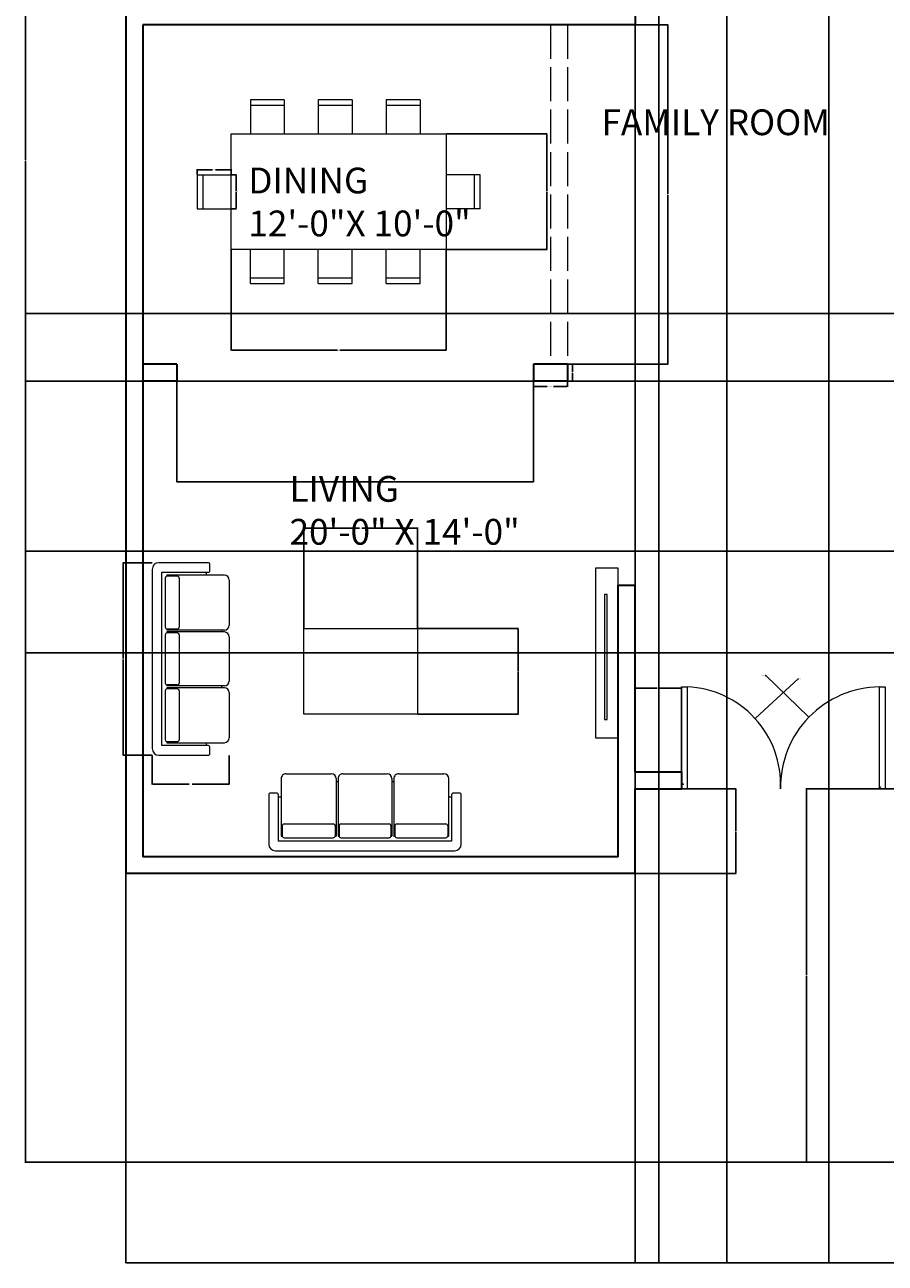
# Model space of a CAD drawing. Units: inches. Extents: x 4468 to 4972, y 2758 to 3538.
# Tile 1 of 4: x 4468 to 4772, y 2758 to 3196. Entities that reach past the tile are written whole.
import ezdxf

# ---------------------------------------------------------------- set-up
doc = ezdxf.new("R2010")
doc.units = ezdxf.units.IN
doc.linetypes.add('ACAD_ISO02W100', pattern=[15, 12, -3])
for name, color, linetype, lineweight in [('A-ANNO-DIMS', 2, 'Continuous', 18), ('A-AREA-IDEN', 7, 'Continuous', 18), ('A-COLS', 7, 'Continuous', 35), ('A-DOOR', 4, 'Continuous', 18), ('A-EQPM', 8, 'Continuous', 18), ('A-FLOR-OVHD', 8, 'ACAD_ISO02W100', 13), ('A-FURN', 8, 'Continuous', 15), ('A-WALL', 7, 'Continuous', 35)]:
    doc.layers.add(name, color=color, linetype=linetype, lineweight=lineweight)
doc.styles.get("Standard").update_dxf_attribs({"font": 'arial.ttf'})
doc.dimstyles.get("Standard").update_dxf_attribs({"dimtxt": 0.18, "dimasz": 0.18, "dimexe": 0.18, "dimexo": 0.0625, "dimgap": 0.09, "dimtad": 0, "dimtih": 1, "dimtoh": 1, "dimdec": 4, "dimzin": 0, "dimdsep": 46, "dimtxsty": 'Standard', "dimcen": 0.09, "dimadec": 0, "dimazin": 0, "dimtfac": 1, "dimtdec": 4, "dimtofl": 0, "dimtmove": 0, "dimatfit": 3, "dimfxl": 1, "dimtolj": 1, "dimtzin": 0, "dimarcsym": 0})

# ---------------------------------------------------------------- blocks, each defined once
blk = doc.blocks.new('A$C06FC73D7')
for p, q in [((1.93, 0.8), (0.07, 0.8)), ((0, 0.73), (0, 0.22)), ((0.1, 0.22), (0.1, 0.7)), ((0.1, 0.7), (1.9, 0.7)), ((0.13, 0.648), (0.13, 0.05)), ((0.14, 0.648), (0.13, 0.648)), ((0.14, 0.54), (0.14, 0.644)), ((0.67, 0.664), (0.16, 0.664)), ((0.7, 0.648), (0.69, 0.648)), ((0.69, 0.54), (0.69, 0.644)), ((0.7, 0.05), (0.7, 0.648)), ((0.72, 0.05), (0.72, 0.648)), ((0.73, 0.648), (0.72, 0.648)), ((0.73, 0.54), (0.73, 0.644)), ((1.25, 0.664), (0.75, 0.664)), ((1.28, 0.648), (1.27, 0.648)), ((1.27, 0.54), (1.27, 0.644)), ((1.28, 0.05), (1.28, 0.648)), ((1.3, 0.05), (1.3, 0.648)), ((1.31, 0.648), (1.3, 0.648)), ((1.31, 0.54), (1.31, 0.644)), ((1.84, 0.664), (1.33, 0.664)), ((1.87, 0.648), (1.86, 0.648)), ((1.86, 0.54), (1.86, 0.644)), ((1.87, 0.05), (1.87, 0.648)), ((1.9, 0.7), (1.9, 0.22)), ((2, 0.22), (2, 0.73)), ((0.67, 0.52), (0.16, 0.52)), ((1.25, 0.52), (0.75, 0.52)), ((1.84, 0.52), (1.33, 0.52)), ((0.02, 0.2), (0.08, 0.2)), ((0.13, 0.24), (0.1, 0.24)), ((1.9, 0.24), (1.87, 0.24)), ((1.92, 0.2), (1.98, 0.2)), ((0.65, 0), (0.18, 0)), ((0.72, 0.08), (0.7, 0.08)), ((1.23, 0), (0.77, 0)), ((1.3, 0.08), (1.28, 0.08)), ((1.82, 0), (1.35, 0))]:
    blk.add_line(p, q)
for centre, radius, start, end in [((0.07, 0.73), 0.07, 90, 180), ((1.93, 0.73), 0.07, 0, 90), ((0.16, 0.644), 0.02, 90, 180), ((0.67, 0.644), 0.02, 0, 90), ((0.75, 0.644), 0.02, 90, 180), ((1.25, 0.644), 0.02, 0, 90), ((1.33, 0.644), 0.02, 90, 180), ((1.84, 0.644), 0.02, 0, 90), ((0.16, 0.54), 0.02, 180, 270), ((0.67, 0.54), 0.02, 270, 0), ((0.75, 0.54), 0.02, 180, 270), ((1.25, 0.54), 0.02, 270, 0), ((1.33, 0.54), 0.02, 180, 270), ((1.84, 0.54), 0.02, 270, 0), ((0.02, 0.22), 0.02, 180, 270), ((0.08, 0.22), 0.02, 270, 0), ((1.92, 0.22), 0.02, 180, 270), ((1.98, 0.22), 0.02, 270, 0), ((0.18, 0.05), 0.05, 180, 270), ((0.65, 0.05), 0.05, 270, 0), ((0.77, 0.05), 0.05, 180, 270), ((1.23, 0.05), 0.05, 270, 0), ((1.35, 0.05), 0.05, 180, 270), ((1.82, 0.05), 0.05, 270, 0)]:
    blk.add_arc(centre, radius, start, end)
blk = doc.blocks.new('CHAIR-DINING')
for p, q in [((0, 0), (0, 12)), ((12, 0), (12, 12)), ((0, 2), (12, 2)), ((0, 0), (12, 0))]:
    blk.add_line(p, q)
blk = doc.blocks.new('COL-12X6')
for p, q in [((12, 6), (0, 6)), ((0, 6), (0, 0)), ((12, 6), (12, 0)), ((12, 0), (0, 0))]:
    blk.add_line(p, q)
blk = doc.blocks.new('DOOR-LEAF-36IN')
for p, q in [((0, 0), (0, 36)), ((0, 36), (2, 36)), ((2, 36), (2, 0)), ((2, 0), (0, 0))]:
    blk.add_line(p, q)
blk = doc.blocks.new('*D15')
at = {"layer": 'A-ANNO-DIMS', "color": 0, "lineweight": -2, "transparency": 16777216}
for p, q in [((4541.41, 3143.14), (4543.32, 3143.14)), ((4543.14, 3142.96), (4543.14, 3137.32)), ((4543.14, 3131.32), (4543.14, 3136.96)), ((4541.41, 3131.14), (4543.32, 3131.14))]:
    blk.add_line(p, q, dxfattribs=at)
at = {"layer": 'A-ANNO-DIMS', "color": 0, "transparency": 16777216}
for points in [[(4543.11, 3142.96), (4543.17, 3142.96), (4543.14, 3143.14)], [(4543.11, 3131.32), (4543.17, 3131.32), (4543.14, 3131.14)]]:
    blk.add_solid(points, dxfattribs=at)
at = {"layer": 'Defpoints', "color": 0, "transparency": 16777216}
for p in [(4541.34, 3143.14), (4541.34, 3131.14), (4543.14, 3131.14)]:
    blk.add_point(p, dxfattribs=at)
at = {"layer": 'A-ANNO-DIMS', "color": 0, "transparency": 16777216, "insert": (4543.14, 3137.14), "char_height": 0.18, "attachment_point": 5}
blk.add_mtext('\\A1;CHAIR 12 TYP.', dxfattribs=at)
blk = doc.blocks.new('*D16')
at = {"layer": 'A-ANNO-DIMS', "color": 0, "lineweight": -2, "transparency": 16777216}
for p, q in [((4529.34, 3143.2), (4529.34, 3145.12)), ((4529.52, 3144.94), (4534.82, 3144.94)), ((4541.16, 3144.94), (4535.86, 3144.94)), ((4541.34, 3143.2), (4541.34, 3145.12))]:
    blk.add_line(p, q, dxfattribs=at)
at = {"layer": 'A-ANNO-DIMS', "color": 0, "transparency": 16777216}
for points in [[(4529.52, 3144.97), (4529.52, 3144.91), (4529.34, 3144.94)], [(4541.16, 3144.97), (4541.16, 3144.91), (4541.34, 3144.94)]]:
    blk.add_solid(points, dxfattribs=at)
at = {"layer": 'Defpoints', "color": 0, "transparency": 16777216}
for p in [(4529.34, 3143.14), (4541.34, 3144.94), (4541.34, 3143.14)]:
    blk.add_point(p, dxfattribs=at)
at = {"layer": 'A-ANNO-DIMS', "color": 0, "transparency": 16777216, "insert": (4535.34, 3144.94), "char_height": 0.18, "attachment_point": 5}
blk.add_mtext('\\A1;12 TYP.', dxfattribs=at)
blk = doc.blocks.new('*D23')
at = {"layer": 'A-ANNO-DIMS', "color": 0, "lineweight": -2, "transparency": 16777216}
for p, q in [((4513.43, 3006.06), (4503.11, 3006.06)), ((4503.29, 3005.88), (4503.29, 2972.22)), ((4503.29, 2938.2), (4503.29, 2971.85)), ((4513.43, 2938.02), (4503.11, 2938.02))]:
    blk.add_line(p, q, dxfattribs=at)
at = {"layer": 'A-ANNO-DIMS', "color": 0, "transparency": 16777216}
for points in [[(4503.26, 3005.88), (4503.32, 3005.88), (4503.29, 3006.06)], [(4503.26, 2938.2), (4503.32, 2938.2), (4503.29, 2938.02)]]:
    blk.add_solid(points, dxfattribs=at)
at = {"layer": 'Defpoints', "color": 0, "transparency": 16777216}
for p in [(4503.29, 3006.06), (4513.49, 3006.06), (4513.49, 2938.02)]:
    blk.add_point(p, dxfattribs=at)
at = {"layer": 'A-ANNO-DIMS', "color": 0, "transparency": 16777216, "insert": (4503.29, 2972.04), "char_height": 0.18, "attachment_point": 5}
blk.add_mtext('\\A1;SOFA 68 TYP.', dxfattribs=at)
blk = doc.blocks.new('*D24')
at = {"layer": 'A-ANNO-DIMS', "color": 0, "lineweight": -2, "transparency": 16777216}
for p, q in [((4513.49, 2937.96), (4513.49, 2927.63)), ((4540.71, 2937.96), (4540.71, 2927.63)), ((4513.67, 2927.81), (4526.57, 2927.81)), ((4540.53, 2927.81), (4527.63, 2927.81))]:
    blk.add_line(p, q, dxfattribs=at)
at = {"layer": 'A-ANNO-DIMS', "color": 0, "transparency": 16777216}
for points in [[(4513.67, 2927.84), (4513.67, 2927.78), (4513.49, 2927.81)], [(4540.53, 2927.84), (4540.53, 2927.78), (4540.71, 2927.81)]]:
    blk.add_solid(points, dxfattribs=at)
at = {"layer": 'Defpoints', "color": 0, "transparency": 16777216}
for p in [(4513.49, 2938.02), (4540.71, 2938.02), (4513.49, 2927.81)]:
    blk.add_point(p, dxfattribs=at)
at = {"layer": 'A-ANNO-DIMS', "color": 0, "transparency": 16777216, "insert": (4527.1, 2927.81), "char_height": 0.18, "attachment_point": 5}
blk.add_mtext('\\A1;27 TYP.', dxfattribs=at)
blk = doc.blocks.new('*D27')
at = {"layer": 'A-ANNO-DIMS', "color": 0, "lineweight": -2, "transparency": 16777216}
for p, q in [((4648.18, 3070.1), (4648.18, 3068.18)), ((4648.36, 3068.36), (4653.07, 3068.36)), ((4660, 3068.36), (4655.28, 3068.36)), ((4660.18, 3070.1), (4660.18, 3068.18))]:
    blk.add_line(p, q, dxfattribs=at)
at = {"layer": 'A-ANNO-DIMS', "color": 0, "transparency": 16777216}
for points in [[(4648.36, 3068.39), (4648.36, 3068.33), (4648.18, 3068.36)], [(4660, 3068.39), (4660, 3068.33), (4660.18, 3068.36)]]:
    blk.add_solid(points, dxfattribs=at)
at = {"layer": 'Defpoints', "color": 0, "transparency": 16777216}
for p in [(4648.18, 3070.16), (4660.18, 3070.16), (4660.18, 3068.36)]:
    blk.add_point(p, dxfattribs=at)
at = {"layer": 'A-ANNO-DIMS', "color": 0, "transparency": 16777216, "insert": (4654.18, 3068.36), "char_height": 0.18, "attachment_point": 5}
blk.add_mtext('\\A1;COLUMN 12 TYP.', dxfattribs=at)
blk = doc.blocks.new('*D28')
at = {"layer": 'A-ANNO-DIMS', "color": 0, "lineweight": -2, "transparency": 16777216}
for p, q in [((4660.24, 3076.16), (4662.16, 3076.16)), ((4661.98, 3075.98), (4661.98, 3073.34)), ((4661.98, 3070.34), (4661.98, 3072.98)), ((4660.24, 3070.16), (4662.16, 3070.16))]:
    blk.add_line(p, q, dxfattribs=at)
at = {"layer": 'A-ANNO-DIMS', "color": 0, "transparency": 16777216}
for points in [[(4661.95, 3075.98), (4662.01, 3075.98), (4661.98, 3076.16)], [(4661.95, 3070.34), (4662.01, 3070.34), (4661.98, 3070.16)]]:
    blk.add_solid(points, dxfattribs=at)
at = {"layer": 'Defpoints', "color": 0, "transparency": 16777216}
for p in [(4660.18, 3076.16), (4661.98, 3076.16), (4660.18, 3070.16)]:
    blk.add_point(p, dxfattribs=at)
at = {"layer": 'A-ANNO-DIMS', "color": 0, "transparency": 16777216, "insert": (4661.98, 3073.16), "char_height": 0.18, "attachment_point": 5}
blk.add_mtext('\\A1;6 TYP.', dxfattribs=at)
blk = doc.blocks.new('*D37')
at = {"layer": 'A-ANNO-DIMS', "color": 0, "lineweight": -2, "transparency": 16777216}
for p, q in [((4504.18, 2896.1), (4504.18, 2758.48)), ((4936.18, 2794.1), (4936.18, 2758.48)), ((4504.36, 2758.66), (4719.88, 2758.66)), ((4936, 2758.66), (4720.47, 2758.66))]:
    blk.add_line(p, q, dxfattribs=at)
at = {"layer": 'A-ANNO-DIMS', "color": 0, "transparency": 16777216}
for points in [[(4504.36, 2758.69), (4504.36, 2758.63), (4504.18, 2758.66)], [(4936, 2758.69), (4936, 2758.63), (4936.18, 2758.66)]]:
    blk.add_solid(points, dxfattribs=at)
at = {"layer": 'Defpoints', "color": 0, "transparency": 16777216}
for p in [(4504.18, 2896.16), (4936.18, 2794.16), (4936.18, 2758.66)]:
    blk.add_point(p, dxfattribs=at)
at = {"layer": 'A-ANNO-DIMS', "color": 0, "transparency": 16777216, "insert": (4720.18, 2758.66), "char_height": 0.18, "attachment_point": 5}
blk.add_mtext('\\A1;432', dxfattribs=at)
blk = doc.blocks.new('*D38')
at = {"layer": 'A-ANNO-DIMS', "color": 0, "lineweight": -2, "transparency": 16777216}
for p, q in [((4504.11, 3502.16), (4468.5, 3502.16)), ((4468.68, 3501.98), (4468.68, 3148.34)), ((4468.68, 2794.34), (4468.68, 3147.98)), ((4780.11, 2794.16), (4468.5, 2794.16))]:
    blk.add_line(p, q, dxfattribs=at)
at = {"layer": 'A-ANNO-DIMS', "color": 0, "transparency": 16777216}
for points in [[(4468.65, 3501.98), (4468.71, 3501.98), (4468.68, 3502.16)], [(4468.65, 2794.34), (4468.71, 2794.34), (4468.68, 2794.16)]]:
    blk.add_solid(points, dxfattribs=at)
at = {"layer": 'Defpoints', "color": 0, "transparency": 16777216}
for p in [(4468.68, 3502.16), (4504.18, 3502.16), (4780.18, 2794.16)]:
    blk.add_point(p, dxfattribs=at)
at = {"layer": 'A-ANNO-DIMS', "color": 0, "transparency": 16777216, "insert": (4468.68, 3148.16), "char_height": 0.18, "attachment_point": 5}
blk.add_mtext('\\A1;708', dxfattribs=at)
blk = doc.blocks.new('*D41')
at = {"layer": 'A-ANNO-DIMS', "color": 0, "lineweight": -2, "transparency": 16777216}
for p, q in [((4684.24, 2926.16), (4719.86, 2926.16)), ((4719.68, 2925.98), (4719.68, 2911.34)), ((4719.68, 2896.34), (4719.68, 2910.98)), ((4684.24, 2896.16), (4719.86, 2896.16))]:
    blk.add_line(p, q, dxfattribs=at)
at = {"layer": 'A-ANNO-DIMS', "color": 0, "transparency": 16777216}
for points in [[(4719.65, 2925.98), (4719.71, 2925.98), (4719.68, 2926.16)], [(4719.65, 2896.34), (4719.71, 2896.34), (4719.68, 2896.16)]]:
    blk.add_solid(points, dxfattribs=at)
at = {"layer": 'Defpoints', "color": 0, "transparency": 16777216}
for p in [(4684.18, 2926.16), (4684.18, 2896.16), (4719.68, 2896.16)]:
    blk.add_point(p, dxfattribs=at)
at = {"layer": 'A-ANNO-DIMS', "color": 0, "transparency": 16777216, "insert": (4719.68, 2911.16), "char_height": 0.18, "attachment_point": 5}
blk.add_mtext('\\A1;30', dxfattribs=at)
blk = doc.blocks.new('*D42')
at = {"layer": 'A-ANNO-DIMS', "color": 0, "lineweight": -2, "transparency": 16777216}
for p, q in [((4780.11, 2926.16), (4744.5, 2926.16)), ((4744.68, 2925.98), (4744.68, 2860.34)), ((4744.68, 2794.34), (4744.68, 2859.98)), ((4780.11, 2794.16), (4744.5, 2794.16))]:
    blk.add_line(p, q, dxfattribs=at)
at = {"layer": 'A-ANNO-DIMS', "color": 0, "transparency": 16777216}
for points in [[(4744.65, 2925.98), (4744.71, 2925.98), (4744.68, 2926.16)], [(4744.65, 2794.34), (4744.71, 2794.34), (4744.68, 2794.16)]]:
    blk.add_solid(points, dxfattribs=at)
at = {"layer": 'Defpoints', "color": 0, "transparency": 16777216}
for p in [(4744.68, 2926.16), (4780.18, 2926.16), (4780.18, 2794.16)]:
    blk.add_point(p, dxfattribs=at)
at = {"layer": 'A-ANNO-DIMS', "color": 0, "transparency": 16777216, "insert": (4744.68, 2860.16), "char_height": 0.18, "attachment_point": 5}
blk.add_mtext('\\A1;132', dxfattribs=at)
blk = doc.blocks.new('*D49')
at = {"layer": 'A-ANNO-DIMS', "color": 0, "lineweight": -2, "transparency": 16777216}
for p, q in [((4522.18, 3070.1), (4522.18, 3034.48)), ((4648.18, 3070.1), (4648.18, 3034.48)), ((4522.36, 3034.66), (4584.9, 3034.66)), ((4648, 3034.66), (4585.46, 3034.66))]:
    blk.add_line(p, q, dxfattribs=at)
at = {"layer": 'A-ANNO-DIMS', "color": 0, "transparency": 16777216}
for points in [[(4522.36, 3034.69), (4522.36, 3034.63), (4522.18, 3034.66)], [(4648, 3034.69), (4648, 3034.63), (4648.18, 3034.66)]]:
    blk.add_solid(points, dxfattribs=at)
at = {"layer": 'Defpoints', "color": 0, "transparency": 16777216}
for p in [(4522.18, 3070.16), (4648.18, 3070.16), (4522.18, 3034.66)]:
    blk.add_point(p, dxfattribs=at)
at = {"layer": 'A-ANNO-DIMS', "color": 0, "transparency": 16777216, "insert": (4585.18, 3034.66), "char_height": 0.18, "attachment_point": 5}
blk.add_mtext('\\A1;126', dxfattribs=at)
blk = doc.blocks.new('*D50')
at = {"layer": 'A-ANNO-DIMS', "color": 0, "lineweight": -2, "transparency": 16777216}
for p, q in [((4660.24, 3196.16), (4695.86, 3196.16)), ((4695.68, 3195.98), (4695.68, 3136.34)), ((4695.68, 3076.34), (4695.68, 3135.98)), ((4660.24, 3076.16), (4695.86, 3076.16))]:
    blk.add_line(p, q, dxfattribs=at)
at = {"layer": 'A-ANNO-DIMS', "color": 0, "transparency": 16777216}
for points in [[(4695.65, 3195.98), (4695.71, 3195.98), (4695.68, 3196.16)], [(4695.65, 3076.34), (4695.71, 3076.34), (4695.68, 3076.16)]]:
    blk.add_solid(points, dxfattribs=at)
at = {"layer": 'Defpoints', "color": 0, "transparency": 16777216}
for p in [(4660.18, 3196.16), (4660.18, 3076.16), (4695.68, 3076.16)]:
    blk.add_point(p, dxfattribs=at)
at = {"layer": 'A-ANNO-DIMS', "color": 0, "transparency": 16777216, "insert": (4695.68, 3136.16), "char_height": 0.18, "attachment_point": 5}
blk.add_mtext('\\A1;120', dxfattribs=at)
blk = doc.blocks.new('*D51')
at = {"layer": 'A-ANNO-DIMS', "color": 0, "lineweight": -2, "transparency": 16777216}
for p, q in [((4541.34, 3116.65), (4541.34, 3081.03)), ((4617.41, 3116.65), (4617.41, 3081.03)), ((4541.52, 3081.21), (4578.98, 3081.21)), ((4617.23, 3081.21), (4579.77, 3081.21))]:
    blk.add_line(p, q, dxfattribs=at)
at = {"layer": 'A-ANNO-DIMS', "color": 0, "transparency": 16777216}
for points in [[(4541.52, 3081.24), (4541.52, 3081.18), (4541.34, 3081.21)], [(4617.23, 3081.24), (4617.23, 3081.18), (4617.41, 3081.21)]]:
    blk.add_solid(points, dxfattribs=at)
at = {"layer": 'Defpoints', "color": 0, "transparency": 16777216}
for p in [(4541.34, 3116.71), (4617.41, 3116.71), (4541.34, 3081.21)]:
    blk.add_point(p, dxfattribs=at)
at = {"layer": 'A-ANNO-DIMS', "color": 0, "transparency": 16777216, "insert": (4579.38, 3081.21), "char_height": 0.18, "attachment_point": 5}
blk.add_mtext('\\A1;76.06', dxfattribs=at)
blk = doc.blocks.new('*D52')
at = {"layer": 'A-ANNO-DIMS', "color": 0, "lineweight": -2, "transparency": 16777216}
for p, q in [((4617.47, 3157.57), (4653.09, 3157.57)), ((4652.91, 3157.39), (4652.91, 3137.32)), ((4652.91, 3116.89), (4652.91, 3136.96)), ((4617.47, 3116.71), (4653.09, 3116.71))]:
    blk.add_line(p, q, dxfattribs=at)
at = {"layer": 'A-ANNO-DIMS', "color": 0, "transparency": 16777216}
for points in [[(4652.88, 3157.39), (4652.94, 3157.39), (4652.91, 3157.57)], [(4652.88, 3116.89), (4652.94, 3116.89), (4652.91, 3116.71)]]:
    blk.add_solid(points, dxfattribs=at)
at = {"layer": 'Defpoints', "color": 0, "transparency": 16777216}
for p in [(4617.41, 3157.57), (4617.41, 3116.71), (4652.91, 3116.71)]:
    blk.add_point(p, dxfattribs=at)
at = {"layer": 'A-ANNO-DIMS', "color": 0, "transparency": 16777216, "insert": (4652.91, 3137.14), "char_height": 0.18, "attachment_point": 5}
blk.add_mtext('\\A1;40.865', dxfattribs=at)
blk = doc.blocks.new('*D53')
at = {"layer": 'A-ANNO-DIMS', "color": 0, "lineweight": -2, "transparency": 16777216}
for p, q in [((4567.05, 2982.83), (4567.05, 3018.45)), ((4567.23, 3018.27), (4586.77, 3018.27)), ((4607.1, 3018.27), (4587.56, 3018.27)), ((4607.28, 2982.83), (4607.28, 3018.45))]:
    blk.add_line(p, q, dxfattribs=at)
at = {"layer": 'A-ANNO-DIMS', "color": 0, "transparency": 16777216}
for points in [[(4567.23, 3018.3), (4567.23, 3018.24), (4567.05, 3018.27)], [(4607.1, 3018.3), (4607.1, 3018.24), (4607.28, 3018.27)]]:
    blk.add_solid(points, dxfattribs=at)
at = {"layer": 'Defpoints', "color": 0, "transparency": 16777216}
for p in [(4607.28, 3018.27), (4567.05, 2982.77), (4607.28, 2982.77)]:
    blk.add_point(p, dxfattribs=at)
at = {"layer": 'A-ANNO-DIMS', "color": 0, "transparency": 16777216, "insert": (4587.16, 3018.27), "char_height": 0.18, "attachment_point": 5}
blk.add_mtext('\\A1;40.23', dxfattribs=at)
blk = doc.blocks.new('*D54')
at = {"layer": 'A-ANNO-DIMS', "color": 0, "lineweight": -2, "transparency": 16777216}
for p, q in [((4607.34, 2982.77), (4642.96, 2982.77)), ((4642.78, 2982.59), (4642.78, 2967.85)), ((4642.78, 2952.74), (4642.78, 2967.48)), ((4607.34, 2952.56), (4642.96, 2952.56))]:
    blk.add_line(p, q, dxfattribs=at)
at = {"layer": 'A-ANNO-DIMS', "color": 0, "transparency": 16777216}
for points in [[(4642.75, 2982.59), (4642.81, 2982.59), (4642.78, 2982.77)], [(4642.75, 2952.74), (4642.81, 2952.74), (4642.78, 2952.56)]]:
    blk.add_solid(points, dxfattribs=at)
at = {"layer": 'Defpoints', "color": 0, "transparency": 16777216}
for p in [(4607.28, 2982.77), (4607.28, 2952.56), (4642.78, 2952.56)]:
    blk.add_point(p, dxfattribs=at)
at = {"layer": 'A-ANNO-DIMS', "color": 0, "transparency": 16777216, "insert": (4642.78, 2967.67), "char_height": 0.18, "attachment_point": 5}
blk.add_mtext('\\A1;30.205', dxfattribs=at)
blk = doc.blocks.new('*D55')
at = {"layer": 'A-ANNO-DIMS', "color": 0, "lineweight": -2, "transparency": 16777216}
for p, q in [((4786.11, 3094.16), (4468.5, 3094.16)), ((4468.68, 3093.98), (4468.68, 3082.34)), ((4468.68, 3070.34), (4468.68, 3081.98)), ((4786.11, 3070.16), (4468.5, 3070.16))]:
    blk.add_line(p, q, dxfattribs=at)
at = {"layer": 'A-ANNO-DIMS', "color": 0, "transparency": 16777216}
for points in [[(4468.65, 3093.98), (4468.71, 3093.98), (4468.68, 3094.16)], [(4468.65, 3070.34), (4468.71, 3070.34), (4468.68, 3070.16)]]:
    blk.add_solid(points, dxfattribs=at)
at = {"layer": 'Defpoints', "color": 0, "transparency": 16777216}
for p in [(4468.68, 3094.16), (4786.18, 3094.16), (4786.18, 3070.16)]:
    blk.add_point(p, dxfattribs=at)
at = {"layer": 'A-ANNO-DIMS', "color": 0, "transparency": 16777216, "insert": (4468.68, 3082.16), "char_height": 0.18, "attachment_point": 5}
blk.add_mtext('\\A1;24', dxfattribs=at)
blk = doc.blocks.new('*D56')
at = {"layer": 'A-ANNO-DIMS', "color": 0, "lineweight": -2, "transparency": 16777216}
for p, q in [((4786.11, 3010.16), (4468.5, 3010.16)), ((4468.68, 3009.98), (4468.68, 2992.34)), ((4468.68, 2974.34), (4468.68, 2991.98)), ((4786.11, 2974.16), (4468.5, 2974.16))]:
    blk.add_line(p, q, dxfattribs=at)
at = {"layer": 'A-ANNO-DIMS', "color": 0, "transparency": 16777216}
for points in [[(4468.65, 3009.98), (4468.71, 3009.98), (4468.68, 3010.16)], [(4468.65, 2974.34), (4468.71, 2974.34), (4468.68, 2974.16)]]:
    blk.add_solid(points, dxfattribs=at)
at = {"layer": 'Defpoints', "color": 0, "transparency": 16777216}
for p in [(4468.68, 3010.16), (4786.18, 3010.16), (4786.18, 2974.16)]:
    blk.add_point(p, dxfattribs=at)
at = {"layer": 'A-ANNO-DIMS', "color": 0, "transparency": 16777216, "insert": (4468.68, 2992.16), "char_height": 0.18, "attachment_point": 5}
blk.add_mtext('\\A1;36', dxfattribs=at)
blk = doc.blocks.new('*D64')
at = {"layer": 'A-ANNO-DIMS', "color": 0, "lineweight": -2, "transparency": 16777216}
for p, q in [((4684.18, 2926.22), (4684.18, 2961.84)), ((4684.36, 2961.66), (4691.95, 2961.66)), ((4700.32, 2961.66), (4692.72, 2961.66)), ((4700.5, 2926.22), (4700.5, 2961.84))]:
    blk.add_line(p, q, dxfattribs=at)
at = {"layer": 'A-ANNO-DIMS', "color": 0, "transparency": 16777216}
for points in [[(4684.36, 2961.69), (4684.36, 2961.63), (4684.18, 2961.66)], [(4700.32, 2961.69), (4700.32, 2961.63), (4700.5, 2961.66)]]:
    blk.add_solid(points, dxfattribs=at)
at = {"layer": 'Defpoints', "color": 0, "transparency": 16777216}
for p in [(4700.5, 2961.66), (4684.18, 2926.16), (4700.5, 2926.16)]:
    blk.add_point(p, dxfattribs=at)
at = {"layer": 'A-ANNO-DIMS', "color": 0, "transparency": 16777216, "insert": (4692.34, 2961.66), "char_height": 0.18, "attachment_point": 5}
blk.add_mtext('\\A1;16.32', dxfattribs=at)
blk = doc.blocks.new('*D66')
at = {"layer": 'A-ANNO-DIMS', "color": 0, "lineweight": -2, "transparency": 16777216}
for p, q in [((4684.18, 3394.1), (4684.18, 2758.48)), ((4692.55, 3394.1), (4692.55, 2758.48)), ((4684.36, 2758.66), (4687.97, 2758.66)), ((4692.37, 2758.66), (4688.76, 2758.66))]:
    blk.add_line(p, q, dxfattribs=at)
at = {"layer": 'A-ANNO-DIMS', "color": 0, "transparency": 16777216}
for points in [[(4684.36, 2758.69), (4684.36, 2758.63), (4684.18, 2758.66)], [(4692.37, 2758.69), (4692.37, 2758.63), (4692.55, 2758.66)]]:
    blk.add_solid(points, dxfattribs=at)
at = {"layer": 'Defpoints', "color": 0, "transparency": 16777216}
for p in [(4684.18, 3394.16), (4692.55, 3394.16), (4692.55, 2758.66)]:
    blk.add_point(p, dxfattribs=at)
at = {"layer": 'A-ANNO-DIMS', "color": 0, "transparency": 16777216, "insert": (4688.36, 2758.66), "char_height": 0.18, "attachment_point": 5}
blk.add_mtext('\\A1;8.375', dxfattribs=at)
blk = doc.blocks.new('*D67')
at = {"layer": 'A-ANNO-DIMS', "color": 0, "lineweight": -2, "transparency": 16777216}
for p, q in [((4716.55, 3394.1), (4716.55, 2758.48)), ((4752.55, 3394.1), (4752.55, 2758.48)), ((4716.73, 2758.66), (4734.33, 2758.66)), ((4752.37, 2758.66), (4734.77, 2758.66))]:
    blk.add_line(p, q, dxfattribs=at)
at = {"layer": 'A-ANNO-DIMS', "color": 0, "transparency": 16777216}
for points in [[(4716.73, 2758.69), (4716.73, 2758.63), (4716.55, 2758.66)], [(4752.37, 2758.69), (4752.37, 2758.63), (4752.55, 2758.66)]]:
    blk.add_solid(points, dxfattribs=at)
at = {"layer": 'Defpoints', "color": 0, "transparency": 16777216}
for p in [(4716.55, 3394.16), (4752.55, 3394.16), (4752.55, 2758.66)]:
    blk.add_point(p, dxfattribs=at)
at = {"layer": 'A-ANNO-DIMS', "color": 0, "transparency": 16777216, "insert": (4734.55, 2758.66), "char_height": 0.18, "attachment_point": 5}
blk.add_mtext('\\A1;36', dxfattribs=at)
blk = doc.blocks.new('*D76')
at = {"layer": 'A-ANNO-DIMS', "color": 0, "lineweight": -2, "transparency": 16777216}
for p, q in [((4730.1, 2966.24), (4730.28, 2966.24)), ((4730.28, 2966.24), (4745.37, 2951.57)), ((4770.78, 2926.78), (4770.96, 2926.78)), ((4770.87, 2926.69), (4770.87, 2926.87))]:
    blk.add_line(p, q, dxfattribs=at)
at = {"layer": 'A-ANNO-DIMS', "color": 0, "transparency": 16777216}
blk.add_solid([(4745.39, 2951.59), (4745.35, 2951.55), (4745.5, 2951.44)], dxfattribs=at)
at = {"layer": 'Defpoints', "color": 0, "transparency": 16777216}
for p in [(4745.5, 2951.44), (4770.87, 2926.78)]:
    blk.add_point(p, dxfattribs=at)
at = {"layer": 'A-ANNO-DIMS', "color": 0, "transparency": 16777216, "insert": (4729.55, 2966.24), "char_height": 0.18, "attachment_point": 5}
blk.add_mtext('\\A1;R35.376', dxfattribs=at)
blk = doc.blocks.new('*D80')
at = {"layer": 'A-ANNO-DIMS', "color": 0, "lineweight": -2, "transparency": 16777216}
for p, q in [((4741.71, 2964.98), (4726.61, 2951.14)), ((4741.89, 2964.98), (4741.71, 2964.98)), ((4701, 2927.74), (4701.18, 2927.74)), ((4701.09, 2927.65), (4701.09, 2927.83))]:
    blk.add_line(p, q, dxfattribs=at)
at = {"layer": 'A-ANNO-DIMS', "color": 0, "transparency": 16777216}
blk.add_solid([(4726.59, 2951.16), (4726.63, 2951.12), (4726.48, 2951.02)], dxfattribs=at)
at = {"layer": 'Defpoints', "color": 0, "transparency": 16777216}
for p in [(4726.48, 2951.02), (4701.09, 2927.74)]:
    blk.add_point(p, dxfattribs=at)
at = {"layer": 'A-ANNO-DIMS', "color": 0, "transparency": 16777216, "insert": (4742.44, 2964.98), "char_height": 0.18, "attachment_point": 5}
blk.add_mtext('\\A1;R34.444', dxfattribs=at)

msp = doc.modelspace()

# ---------------------------------------------------------------- linework, layer by layer
at = {"layer": 'A-DOOR'}
for centre, radius, start, end in [((4701.0881, 2927.7425), 34.4445, 357.363717, 87.657177), ((4770.8665, 2926.7843), 35.3758, 90.59977, 181.014089)]:
    msp.add_arc(centre, radius, start, end, dxfattribs=at)
at = {"layer": 'A-EQPM'}
msp.add_lwpolyline([(4674.194, 2994.7549), (4673.2802, 2994.7549), (4673.2802, 2950.656), (4674.194, 2950.656)], close=True, dxfattribs=at)
at = {"layer": 'A-FLOR-OVHD'}
for p, q in [((4654.1753, 3196.1582), (4654.1753, 3076.1582)), ((4660.1753, 3196.1582), (4660.1753, 3076.1582))]:
    msp.add_line(p, q, dxfattribs=at)
at = {"layer": 'A-FURN'}
for p, q in [((4678.1753, 3004.1582), (4670.1753, 3004.1582)), ((4670.1753, 3004.1582), (4670.1753, 2944.1582)), ((4678.1753, 2998.1582), (4678.1753, 3004.1582)), ((4670.1753, 2944.1582), (4678.1753, 2944.1582))]:
    msp.add_line(p, q, dxfattribs=at)
for points in [[(4541.344, 3157.5745), (4617.406, 3157.5745), (4617.406, 3116.7093), (4541.344, 3116.7093)], [(4567.0467, 2982.7688), (4607.2796, 2982.7688), (4607.2796, 2952.5635), (4567.0467, 2952.5635)]]:
    msp.add_lwpolyline(points, close=True, dxfattribs=at)
at = {"layer": 'A-WALL'}
for p, q in [((4504.1753, 3502.1582), (4504.1753, 2896.1582)), ((4684.1753, 3304.5528), (4684.1753, 3196.1582)), ((4684.1753, 3196.1582), (4510.1753, 3196.1582)), ((4510.1753, 3196.1582), (4510.1753, 3076.1582)), ((4510.1753, 3070.1582), (4510.1753, 2902.1582)), ((4678.1753, 2902.1582), (4678.1753, 2998.1582)), ((4678.1753, 2998.1582), (4684.1753, 2998.1582)), ((4684.1753, 2932.1582), (4684.1753, 2998.1582)), ((4684.1753, 2932.1582), (4700.4962, 2932.1582)), ((4700.4962, 2932.1582), (4700.4962, 2926.1582)), ((4684.1753, 2896.1582), (4684.1753, 2926.1582)), ((4684.1753, 2926.1582), (4700.4962, 2926.1582)), ((4678.1753, 2902.1582), (4510.1753, 2902.1582)), ((4684.1753, 2896.1582), (4504.1753, 2896.1582))]:
    msp.add_line(p, q, dxfattribs=at)

# ---------------------------------------------------------------- block references
at = {"layer": 'A-COLS'}
for p in [(4510.1753, 3070.1582), (4648.1753, 3070.1582)]:
    msp.add_blockref('COL-12X6', p, dxfattribs=at)
at = {"layer": 'A-DOOR'}
msp.add_blockref('DOOR-LEAF-36IN', (4700.4962, 2926.1582), dxfattribs=at)
at = {"layer": 'A-DOOR', "rotation": 180}
msp.add_blockref('DOOR-LEAF-36IN', (4772.4962, 2962.1582), dxfattribs=at)
at = {"layer": 'A-FURN'}
for p, rotation in [((4560.171, 3169.5745), 180), ((4584.171, 3169.5745), 180), ((4608.171, 3169.5745), 180), ((4529.344, 3143.1419), 269.999999999998), ((4629.406, 3131.1419), 89.999999999998)]:
    msp.add_blockref('CHAIR-DINING', p, dxfattribs=dict(at, rotation=rotation))
for p in [(4548.171, 3104.7093), (4572.171, 3104.7093), (4596.171, 3104.7093)]:
    msp.add_blockref('CHAIR-DINING', p, dxfattribs=at)
at = {"layer": 'A-FURN', "xscale": 34.01988650470097, "yscale": 34.01988650470097, "zscale": 34.01988650470097}
for p, rotation in [((4540.7107, 2938.0177), 90), ((4622.7046, 2931.435), 180)]:
    msp.add_blockref('A$C06FC73D7', p, dxfattribs=dict(at, rotation=rotation))

# ---------------------------------------------------------------- texts
at = {"layer": 'A-AREA-IDEN', "char_height": 9.103585, "attachment_point": 1}
for s, insert in [('FAMILY ROOM ', (4672.2504, 3166.2465)), ('DINING\\P12\'-0"X 10\'-0"', (4547.4785, 3145.6724)), ('LIVING\\P20\'-0" X 14\'-0"', (4562.017, 3036.6924))]:
    msp.add_mtext_dynamic_manual_height_columns(s, width=327.642018, gutter_width=45.5179, heights=[0], dxfattribs=dict(at, insert=insert))

# ---------------------------------------------------------------- dimensions: what is measured, and where the dimension line sits
at = {"layer": 'A-ANNO-DIMS'}
for base, p1, p2, angle, override, picture, middle in [((4468.6753, 3502.1582), (4780.1753, 2794.1582), (4504.1753, 3502.1582), 90, {"dimdec": 0, "dimlfac": 1, "dimrnd": 0, "dimzin": 0, "dimdsep": 46, "dimlunit": 2}, '*D38', (4468.6753, 3148.1582)), ((4695.6753, 3076.1582), (4660.1753, 3196.1582), (4660.1753, 3076.1582), 270, {"dimdec": 0, "dimlfac": 1, "dimrnd": 0, "dimzin": 0, "dimdsep": 46, "dimlunit": 2}, '*D50', (4695.6753, 3136.1582)), ((4652.906, 3116.7093), (4617.406, 3157.5745), (4617.406, 3116.7093), 270, {"dimdec": 3, "dimlfac": 1, "dimrnd": 0, "dimzin": 0, "dimdsep": 46, "dimlunit": 2}, '*D52', (4652.906, 3137.1419)), ((4541.344, 3081.2093), (4617.406, 3116.7093), (4541.344, 3116.7093), 180, {"dimdec": 2, "dimlfac": 1, "dimrnd": 0, "dimzin": 0, "dimdsep": 46, "dimlunit": 2}, '*D51', (4579.375, 3081.2093)), ((4468.6753, 3094.1582), (4786.1753, 3070.1582), (4786.1753, 3094.1582), 90, {"dimdec": 0, "dimlfac": 1, "dimrnd": 0, "dimzin": 0, "dimdsep": 46, "dimlunit": 2}, '*D55', (4468.6753, 3082.1582)), ((4522.1753, 3034.6582), (4648.1753, 3070.1582), (4522.1753, 3070.1582), 180, {"dimdec": 0, "dimlfac": 1, "dimrnd": 0, "dimzin": 0, "dimdsep": 46, "dimlunit": 2}, '*D49', (4585.1753, 3034.6582)), ((4468.6753, 3010.1582), (4786.1753, 2974.1582), (4786.1753, 3010.1582), 90, {"dimdec": 0, "dimlfac": 1, "dimrnd": 0, "dimzin": 0, "dimdsep": 46, "dimlunit": 2}, '*D56', (4468.6753, 2992.1582)), ((4642.7796, 2952.5635), (4607.2796, 2982.7688), (4607.2796, 2952.5635), 270, {"dimdec": 3, "dimlfac": 1, "dimrnd": 0, "dimzin": 0, "dimdsep": 46, "dimlunit": 2}, '*D54', (4642.7796, 2967.6661)), ((4719.6753, 2896.1582), (4684.1753, 2926.1582), (4684.1753, 2896.1582), 270, {"dimdec": 0, "dimlfac": 1, "dimrnd": 0, "dimzin": 0, "dimdsep": 46, "dimlunit": 2}, '*D41', (4719.6753, 2911.1582)), ((4744.6753, 2926.1582), (4780.1753, 2794.1582), (4780.1753, 2926.1582), 90, {"dimdec": 0, "dimlfac": 1, "dimrnd": 0, "dimzin": 0, "dimdsep": 46, "dimlunit": 2}, '*D42', (4744.6753, 2860.1582))]:
    dim = msp.add_linear_dim(base=base, p1=p1, p2=p2, angle=angle, dimstyle='Standard', override=override, dxfattribs=at)
    dim.commit()
    dim.dimension.update_dxf_attribs({"geometry": picture, "text_midpoint": middle})
for base, p1, p2, override, picture, middle in [((4692.5504, 2758.6582), (4684.1753, 3394.1582), (4692.5504, 3394.1582), {"dimdec": 3, "dimlfac": 1, "dimrnd": 0, "dimzin": 0, "dimdsep": 46, "dimlunit": 2}, '*D66', (4688.3629, 2758.6582)), ((4752.5504, 2758.6582), (4716.5504, 3394.1582), (4752.5504, 3394.1582), {"dimdec": 0, "dimlfac": 1, "dimrnd": 0, "dimzin": 0, "dimdsep": 46, "dimlunit": 2}, '*D67', (4734.5504, 2758.6582)), ((4607.2796, 3018.2688), (4567.0467, 2982.7688), (4607.2796, 2982.7688), {"dimdec": 2, "dimlfac": 1, "dimrnd": 0, "dimzin": 0, "dimdsep": 46, "dimlunit": 2}, '*D53', (4587.1632, 3018.2688)), ((4700.4962, 2961.6582), (4684.1753, 2926.1582), (4700.4962, 2926.1582), {"dimdec": 2, "dimlfac": 1, "dimrnd": 0, "dimzin": 0, "dimdsep": 46, "dimlunit": 2}, '*D64', (4692.3357, 2961.6582)), ((4936.1753, 2758.6582), (4504.1753, 2896.1582), (4936.1753, 2794.1582), {"dimdec": 0, "dimlfac": 1, "dimrnd": 0, "dimzin": 0, "dimdsep": 46, "dimlunit": 2}, '*D37', (4720.1753, 2758.6582))]:
    dim = msp.add_linear_dim(base=base, p1=p1, p2=p2, dimstyle='Standard', override=override, dxfattribs=at)
    dim.commit()
    dim.dimension.update_dxf_attribs({"geometry": picture, "text_midpoint": middle})
for base, p1, p2, text, picture, middle in [((4541.344, 3144.9419), (4529.344, 3143.1419), (4541.344, 3143.1419), '<> TYP.', '*D16', (4535.344, 3144.9419)), ((4660.1753, 3068.3582), (4648.1753, 3070.1582), (4660.1753, 3070.1582), 'COLUMN <> TYP.', '*D27', (4654.1753, 3068.3582))]:
    dim = msp.add_linear_dim(base=base, p1=p1, p2=p2, text=text, dimstyle='Standard', override={"dimdec": 0, "dimlfac": 1, "dimrnd": 0, "dimzin": 0, "dimdsep": 46, "dimlunit": 2}, dxfattribs=at)
    dim.commit()
    dim.dimension.update_dxf_attribs({"geometry": picture, "text_midpoint": middle})
for base, p1, p2, angle, text, picture, middle in [((4543.144, 3131.1419), (4541.344, 3143.1419), (4541.344, 3131.1419), 270, 'CHAIR <> TYP.', '*D15', (4543.144, 3137.1419)), ((4661.9753, 3076.1582), (4660.1753, 3070.1582), (4660.1753, 3076.1582), 90, '<> TYP.', '*D28', (4661.9753, 3073.1582)), ((4503.2888, 3006.0575), (4513.4948, 2938.0177), (4513.4948, 3006.0575), 90, 'SOFA <> TYP.', '*D23', (4503.2888, 2972.0376)), ((4513.4948, 2927.8118), (4540.7107, 2938.0177), (4513.4948, 2938.0177), 180, '<> TYP.', '*D24', (4527.1027, 2927.8118))]:
    dim = msp.add_linear_dim(base=base, p1=p1, p2=p2, angle=angle, text=text, dimstyle='Standard', override={"dimdec": 0, "dimlfac": 1, "dimrnd": 0, "dimzin": 0, "dimdsep": 46, "dimlunit": 2}, dxfattribs=at)
    dim.commit()
    dim.dimension.update_dxf_attribs({"geometry": picture, "text_midpoint": middle})
for center, mpoint, picture, middle in [((4701.08812, 2927.74253), (4726.47877, 2951.01779), '*D80', (4742.44256, 2964.98295)), ((4770.8665, 2926.7843), (4745.5021, 2951.4439), '*D76', (4729.5537, 2966.2397))]:
    dim = msp.add_radius_dim(center=center, mpoint=mpoint, dimstyle='Standard', override={"dimdec": 3, "dimlfac": 1, "dimrnd": 0, "dimzin": 0, "dimdsep": 46, "dimlunit": 2}, dxfattribs=at)
    dim.commit()
    dim.dimension.update_dxf_attribs({"geometry": picture, "text_midpoint": middle, "dimtype": 164})

doc.saveas('drawing.dxf')
